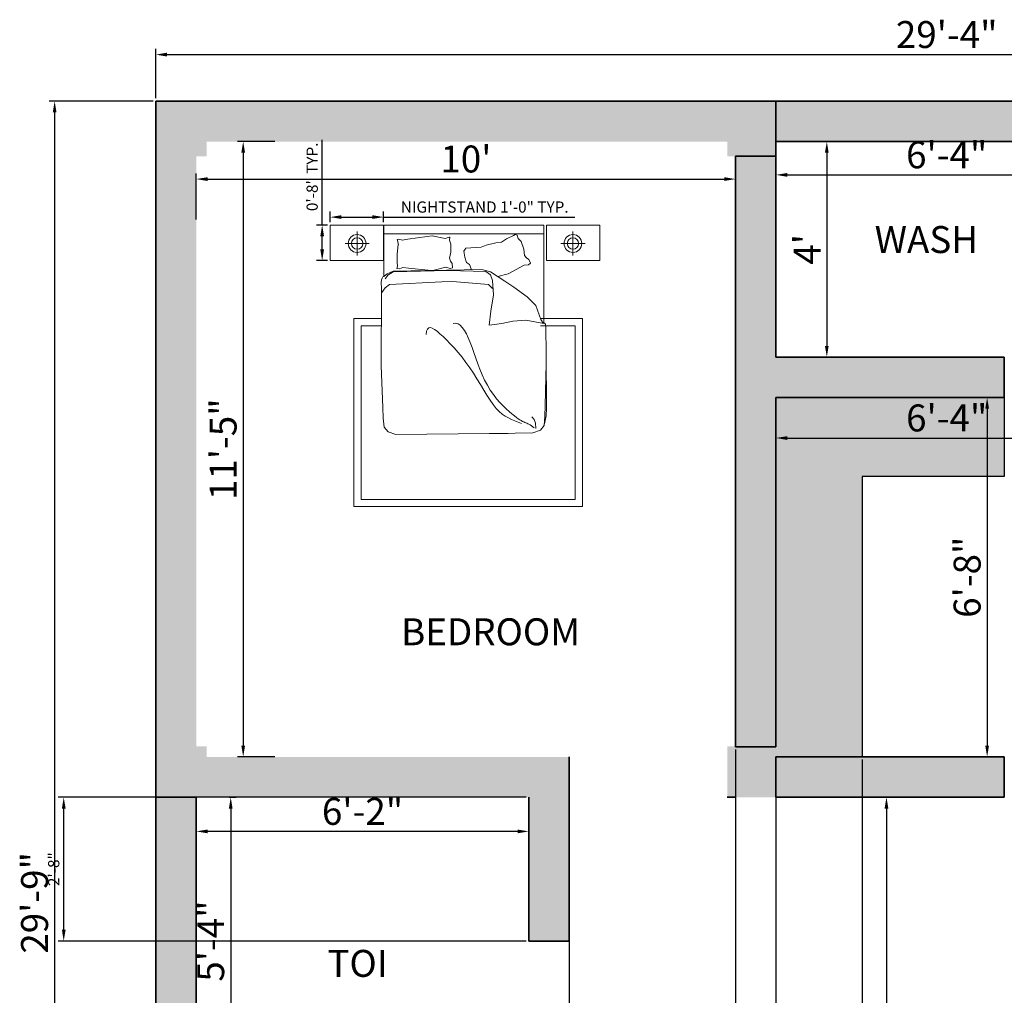
# Model space of a CAD drawing. Units: inches. Extents: x 3025 to 3429, y 1771 to 2198.
# Tile 2 of 3: x 3025 to 3244, y 1981 to 2198. Entities that reach past the tile are written whole.
import ezdxf

# ---------------------------------------------------------------- set-up
doc = ezdxf.new("R2010")
doc.units = ezdxf.units.IN
for name, color, linetype, lineweight in [('A-ANNO-DIMS', 2, 'Continuous', 18), ('A-AREA-IDEN', 7, 'Continuous', 25), ('A-COLS', 7, 'Continuous', 35), ('A-FLOR-FIXT', 9, 'Continuous', 25), ('A-FLOR-FIXT-PATT', 252, 'Continuous', 13), ('A-FURN', 8, 'Continuous', 18), ('A-WALL', 7, 'Continuous', 35), ('A-WALL-PATT', 3, 'Continuous', 13)]:
    doc.layers.add(name, color=color, linetype=linetype, lineweight=lineweight)
doc.layers.add('A-COLS-PATT', color=18, linetype='Continuous', lineweight=13, true_color=0x000000)
doc.styles.get("Standard").update_dxf_attribs({"font": 'arial.ttf'})
doc.dimstyles.new('ISO-25', dxfattribs={"dimtxt": 2.5, "dimasz": 2.5, "dimexe": 1.25, "dimexo": 0.625, "dimtad": 1, "dimdec": 0, "dimlunit": 3, "dimtxsty": 'Standard', "dimcen": 2.5, "dimadec": 0, "dimazin": 0, "dimtfac": 1, "dimtdec": 0, "dimtmove": 0, "dimatfit": 3, "dimfxl": 1, "dimarcsym": 0})

# ---------------------------------------------------------------- blocks, each defined once
blk = doc.blocks.new('*D1')
at = {"layer": 'A-ANNO-DIMS', "color": 0, "lineweight": -2, "transparency": 16777216}
for p, q in [((3054.93, 2180.84), (3054.93, 2191.81)), ((3406.93, 2180.84), (3406.93, 2191.81)), ((3057.43, 2190.56), (3404.43, 2190.56))]:
    blk.add_line(p, q, dxfattribs=at)
at = {"layer": 'A-ANNO-DIMS', "color": 0, "transparency": 16777216}
for points in [[(3057.43, 2190.98), (3057.43, 2190.14), (3054.93, 2190.56)], [(3404.43, 2190.98), (3404.43, 2190.14), (3406.93, 2190.56)]]:
    blk.add_solid(points, dxfattribs=at)
at = {"layer": 'Defpoints', "color": 0, "transparency": 16777216}
for p in [(3406.93, 2190.56), (3054.93, 2180.21), (3406.93, 2180.21)]:
    blk.add_point(p, dxfattribs=at)
at = {"layer": 'A-ANNO-DIMS', "color": 0, "transparency": 16777216, "insert": (3230.93, 2194.25), "char_height": 6, "attachment_point": 5}
blk.add_mtext('29\'-4"', dxfattribs=at)
blk = doc.blocks.new('*D2')
at = {"layer": 'A-ANNO-DIMS', "color": 0, "lineweight": -2, "transparency": 16777216}
for p, q in [((3071.28, 2025.21), (3072.84, 2025.21)), ((3071.59, 2022.71), (3071.59, 1963.71)), ((3071.28, 1961.21), (3072.84, 1961.21))]:
    blk.add_line(p, q, dxfattribs=at)
at = {"layer": 'A-ANNO-DIMS', "color": 0, "transparency": 16777216}
for points in [[(3071.17, 2022.71), (3072, 2022.71), (3071.59, 2025.21)], [(3071.17, 1963.71), (3072, 1963.71), (3071.59, 1961.21)]]:
    blk.add_solid(points, dxfattribs=at)
at = {"layer": 'Defpoints', "color": 0, "transparency": 16777216}
for p in [(3070.66, 2025.21), (3070.66, 1961.21), (3071.59, 1961.21)]:
    blk.add_point(p, dxfattribs=at)
at = {"layer": 'A-ANNO-DIMS', "color": 0, "transparency": 16777216, "insert": (3067.91, 1993.21), "char_height": 6, "attachment_point": 5, "rotation": 90}
blk.add_mtext('5\'-4"', dxfattribs=at)
blk = doc.blocks.new('*D3')
at = {"layer": 'A-ANNO-DIMS', "color": 0, "lineweight": -2, "transparency": 16777216}
for p, q in [((3063.93, 1994.3), (3063.93, 2018.87)), ((3137.93, 2006.87), (3137.93, 2018.87)), ((3135.43, 2017.62), (3066.43, 2017.62))]:
    blk.add_line(p, q, dxfattribs=at)
at = {"layer": 'A-ANNO-DIMS', "color": 0, "transparency": 16777216}
for points in [[(3066.43, 2018.03), (3066.43, 2017.2), (3063.93, 2017.62)], [(3135.43, 2018.03), (3135.43, 2017.2), (3137.93, 2017.62)]]:
    blk.add_solid(points, dxfattribs=at)
at = {"layer": 'Defpoints', "color": 0, "transparency": 16777216}
for p in [(3063.93, 2017.62), (3137.93, 2006.24), (3063.93, 1993.67)]:
    blk.add_point(p, dxfattribs=at)
at = {"layer": 'A-ANNO-DIMS', "color": 0, "transparency": 16777216, "insert": (3100.93, 2021.3), "char_height": 6, "attachment_point": 5}
blk.add_mtext('6\'-2"', dxfattribs=at)
blk = doc.blocks.new('*D6')
at = {"layer": 'A-ANNO-DIMS', "color": 0, "lineweight": -2, "transparency": 16777216}
for p, q in [((3081.41, 2171.21), (3073.12, 2171.21)), ((3074.37, 2168.71), (3074.37, 2036.71)), ((3081.41, 2034.21), (3073.12, 2034.21))]:
    blk.add_line(p, q, dxfattribs=at)
at = {"layer": 'A-ANNO-DIMS', "color": 0, "transparency": 16777216}
for points in [[(3073.95, 2168.71), (3074.78, 2168.71), (3074.37, 2171.21)], [(3073.95, 2036.71), (3074.78, 2036.71), (3074.37, 2034.21)]]:
    blk.add_solid(points, dxfattribs=at)
at = {"layer": 'Defpoints', "color": 0, "transparency": 16777216}
for p in [(3082.03, 2171.21), (3074.37, 2034.21), (3082.03, 2034.21)]:
    blk.add_point(p, dxfattribs=at)
at = {"layer": 'A-ANNO-DIMS', "color": 0, "transparency": 16777216, "insert": (3070.68, 2102.71), "char_height": 6, "attachment_point": 5, "rotation": 90}
blk.add_mtext('11\'-5"', dxfattribs=at)
blk = doc.blocks.new('*D7')
at = {"layer": 'A-ANNO-DIMS', "color": 0, "lineweight": -2, "transparency": 16777216}
for p, q in [((3063.93, 2153.83), (3063.93, 2164.1)), ((3066.43, 2162.85), (3181.43, 2162.85)), ((3183.93, 2145.67), (3183.93, 2164.1))]:
    blk.add_line(p, q, dxfattribs=at)
at = {"layer": 'A-ANNO-DIMS', "color": 0, "transparency": 16777216}
for points in [[(3066.43, 2163.26), (3066.43, 2162.43), (3063.93, 2162.85)], [(3181.43, 2163.26), (3181.43, 2162.43), (3183.93, 2162.85)]]:
    blk.add_solid(points, dxfattribs=at)
at = {"layer": 'Defpoints', "color": 0, "transparency": 16777216}
for p in [(3183.93, 2162.85), (3063.93, 2153.2), (3183.93, 2145.04)]:
    blk.add_point(p, dxfattribs=at)
at = {"layer": 'A-ANNO-DIMS', "color": 0, "transparency": 16777216, "insert": (3123.93, 2166.54), "char_height": 6, "attachment_point": 5}
blk.add_mtext("10'", dxfattribs=at)
blk = doc.blocks.new('*D8')
at = {"layer": 'A-ANNO-DIMS', "color": 0, "lineweight": -2, "transparency": 16777216}
for p, q in [((3205.85, 2171.21), (3203, 2171.21)), ((3204.25, 2168.71), (3204.25, 2125.71)), ((3205.85, 2123.21), (3203, 2123.21))]:
    blk.add_line(p, q, dxfattribs=at)
at = {"layer": 'A-ANNO-DIMS', "color": 0, "transparency": 16777216}
for points in [[(3203.83, 2168.71), (3204.66, 2168.71), (3204.25, 2171.21)], [(3203.83, 2125.71), (3204.66, 2125.71), (3204.25, 2123.21)]]:
    blk.add_solid(points, dxfattribs=at)
at = {"layer": 'Defpoints', "color": 0, "transparency": 16777216}
for p in [(3206.47, 2171.21), (3204.25, 2123.21), (3206.47, 2123.21)]:
    blk.add_point(p, dxfattribs=at)
at = {"layer": 'A-ANNO-DIMS', "color": 0, "transparency": 16777216, "insert": (3200.62, 2147.21), "char_height": 6, "attachment_point": 5, "rotation": 90}
blk.add_mtext("4'", dxfattribs=at)
blk = doc.blocks.new('*D9')
at = {"layer": 'A-ANNO-DIMS', "color": 0, "lineweight": -2, "transparency": 16777216}
for p, q in [((3192.93, 2164.54), (3192.93, 2162.53)), ((3195.43, 2163.78), (3266.43, 2163.78)), ((3268.93, 2164.54), (3268.93, 2162.53))]:
    blk.add_line(p, q, dxfattribs=at)
at = {"layer": 'A-ANNO-DIMS', "color": 0, "transparency": 16777216}
for points in [[(3195.43, 2164.2), (3195.43, 2163.37), (3192.93, 2163.78)], [(3266.43, 2164.2), (3266.43, 2163.37), (3268.93, 2163.78)]]:
    blk.add_solid(points, dxfattribs=at)
at = {"layer": 'Defpoints', "color": 0, "transparency": 16777216}
for p in [(3192.93, 2165.16), (3268.93, 2165.16), (3268.93, 2163.78)]:
    blk.add_point(p, dxfattribs=at)
at = {"layer": 'A-ANNO-DIMS', "color": 0, "transparency": 16777216, "insert": (3230.93, 2167.47), "char_height": 6, "attachment_point": 5}
blk.add_mtext('6\'-4"', dxfattribs=at)
blk = doc.blocks.new('*D12')
at = {"layer": 'A-ANNO-DIMS', "color": 0, "lineweight": -2, "transparency": 16777216}
for p, q in [((3054.31, 2180.21), (3031.16, 2180.21)), ((3032.41, 2177.71), (3032.41, 1825.71)), ((3054.31, 1823.21), (3031.16, 1823.21))]:
    blk.add_line(p, q, dxfattribs=at)
at = {"layer": 'A-ANNO-DIMS', "color": 0, "transparency": 16777216}
for points in [[(3031.99, 2177.71), (3032.82, 2177.71), (3032.41, 2180.21)], [(3031.99, 1825.71), (3032.82, 1825.71), (3032.41, 1823.21)]]:
    blk.add_solid(points, dxfattribs=at)
at = {"layer": 'Defpoints', "color": 0, "transparency": 16777216}
for p in [(3054.93, 2180.21), (3032.41, 1823.21), (3054.93, 1823.21)]:
    blk.add_point(p, dxfattribs=at)
at = {"layer": 'A-ANNO-DIMS', "color": 0, "transparency": 16777216, "insert": (3028.72, 2001.71), "char_height": 6, "attachment_point": 5, "rotation": 90}
blk.add_mtext('29\'-9"', dxfattribs=at)
blk = doc.blocks.new('*D14')
at = {"layer": 'A-ANNO-DIMS', "color": 0, "lineweight": -2, "transparency": 16777216}
for p, q in [((3227.77, 2114.21), (3241.17, 2114.21)), ((3239.92, 2111.71), (3239.92, 2036.71)), ((3227.77, 2034.21), (3241.17, 2034.21))]:
    blk.add_line(p, q, dxfattribs=at)
at = {"layer": 'A-ANNO-DIMS', "color": 0, "transparency": 16777216}
for points in [[(3239.51, 2111.71), (3240.34, 2111.71), (3239.92, 2114.21)], [(3239.51, 2036.71), (3240.34, 2036.71), (3239.92, 2034.21)]]:
    blk.add_solid(points, dxfattribs=at)
at = {"layer": 'Defpoints', "color": 0, "transparency": 16777216}
for p in [(3227.15, 2114.21), (3227.15, 2034.21), (3239.92, 2034.21)]:
    blk.add_point(p, dxfattribs=at)
at = {"layer": 'A-ANNO-DIMS', "color": 0, "transparency": 16777216, "insert": (3236.24, 2074.21), "char_height": 6, "attachment_point": 5, "rotation": 90}
blk.add_mtext('6\'-8"', dxfattribs=at)
blk = doc.blocks.new('*D15')
at = {"layer": 'A-ANNO-DIMS', "color": 0, "lineweight": -2, "transparency": 16777216}
for p, q in [((3192.93, 2097.44), (3192.93, 2106.45)), ((3268.93, 2098.84), (3268.93, 2106.45)), ((3195.43, 2105.2), (3266.43, 2105.2))]:
    blk.add_line(p, q, dxfattribs=at)
at = {"layer": 'A-ANNO-DIMS', "color": 0, "transparency": 16777216}
for points in [[(3195.43, 2105.61), (3195.43, 2104.78), (3192.93, 2105.2)], [(3266.43, 2105.61), (3266.43, 2104.78), (3268.93, 2105.2)]]:
    blk.add_solid(points, dxfattribs=at)
at = {"layer": 'Defpoints', "color": 0, "transparency": 16777216}
for p in [(3268.93, 2105.2), (3268.93, 2098.21), (3192.93, 2096.82)]:
    blk.add_point(p, dxfattribs=at)
at = {"layer": 'A-ANNO-DIMS', "color": 0, "transparency": 16777216, "insert": (3230.93, 2108.89), "char_height": 6, "attachment_point": 5}
blk.add_mtext('6\'-4"', dxfattribs=at)
blk = doc.blocks.new('*D17')
at = {"layer": 'A-ANNO-DIMS', "color": 0, "lineweight": -2, "transparency": 16777216}
for p, q in [((3225.75, 2025.21), (3216.27, 2025.21)), ((3217.52, 2022.71), (3217.52, 1910.71)), ((3225.75, 1908.21), (3216.27, 1908.21))]:
    blk.add_line(p, q, dxfattribs=at)
at = {"layer": 'A-ANNO-DIMS', "color": 0, "transparency": 16777216}
for points in [[(3217.1, 2022.71), (3217.94, 2022.71), (3217.52, 2025.21)], [(3217.1, 1910.71), (3217.94, 1910.71), (3217.52, 1908.21)]]:
    blk.add_solid(points, dxfattribs=at)
at = {"layer": 'Defpoints', "color": 0, "transparency": 16777216}
for p in [(3226.37, 2025.21), (3217.52, 1908.21), (3226.37, 1908.21)]:
    blk.add_point(p, dxfattribs=at)
at = {"layer": 'A-ANNO-DIMS', "color": 0, "transparency": 16777216, "insert": (3213.83, 1966.71), "char_height": 6, "attachment_point": 5, "rotation": 90}
blk.add_mtext('9\'-9"', dxfattribs=at)
blk = doc.blocks.new('NIGHTSTAND-12IN')
for p, q in [((6, 6.52), (6, 1.13)), ((3.31, 3.82), (8.69, 3.82))]:
    blk.add_line(p, q)
blk.add_lwpolyline([(0, 0), (11.88, 0), (11.88, 7.92), (0, 7.92)], close=True)
for radius in [1.98, 1.27]:
    blk.add_circle((6, 3.82), radius)
blk = doc.blocks.new('*D23')
at = {"layer": 'A-ANNO-DIMS', "color": 0, "lineweight": -2, "transparency": 16777216}
for p, q in [((3093.72, 2153.23), (3093.72, 2155.63)), ((3096.22, 2154.38), (3103.1, 2154.38)), ((3105.6, 2153.23), (3105.6, 2155.63)), ((3105.6, 2154.38), (3148.14, 2154.38))]:
    blk.add_line(p, q, dxfattribs=at)
at = {"layer": 'A-ANNO-DIMS', "color": 0, "transparency": 16777216}
for points in [[(3096.22, 2154.8), (3096.22, 2153.97), (3093.72, 2154.38)], [(3103.1, 2154.8), (3103.1, 2153.97), (3105.6, 2154.38)]]:
    blk.add_solid(points, dxfattribs=at)
at = {"layer": 'Defpoints', "color": 0, "transparency": 16777216}
for p in [(3105.6, 2154.38), (3093.72, 2152.6), (3105.6, 2152.6)]:
    blk.add_point(p, dxfattribs=at)
at = {"layer": 'A-ANNO-DIMS', "color": 0, "transparency": 16777216, "insert": (3128.12, 2156.3), "char_height": 2.5, "attachment_point": 5}
blk.add_mtext('NIGHTSTAND 1\'-0" TYP.', dxfattribs=at)
blk = doc.blocks.new('*D24')
at = {"layer": 'A-ANNO-DIMS', "color": 0, "lineweight": -2, "transparency": 16777216}
for p, q in [((3091.94, 2152.6), (3091.94, 2171.59)), ((3093.1, 2152.6), (3090.69, 2152.6)), ((3091.94, 2147.19), (3091.94, 2150.1)), ((3093.1, 2144.69), (3090.69, 2144.69))]:
    blk.add_line(p, q, dxfattribs=at)
at = {"layer": 'A-ANNO-DIMS', "color": 0, "transparency": 16777216}
for points in [[(3091.52, 2150.1), (3092.36, 2150.1), (3091.94, 2152.6)], [(3091.52, 2147.19), (3092.36, 2147.19), (3091.94, 2144.69)]]:
    blk.add_solid(points, dxfattribs=at)
at = {"layer": 'Defpoints', "color": 0, "transparency": 16777216}
for p in [(3091.94, 2152.6), (3093.72, 2152.6), (3093.72, 2144.69)]:
    blk.add_point(p, dxfattribs=at)
at = {"layer": 'A-ANNO-DIMS', "color": 0, "transparency": 16777216, "insert": (3090.04, 2163.35), "char_height": 2.5, "attachment_point": 5, "rotation": 90}
blk.add_mtext('0\'-8" TYP.', dxfattribs=at)
blk = doc.blocks.new('*D37')
at = {"layer": 'A-ANNO-DIMS', "color": 0, "lineweight": -2, "transparency": 16777216}
for p, q in [((3183.93, 2035.84), (3183.93, 1771.46)), ((3146.93, 2033.59), (3146.93, 1771.46)), ((3149.43, 1772.71), (3181.43, 1772.71))]:
    blk.add_line(p, q, dxfattribs=at)
at = {"layer": 'A-ANNO-DIMS', "color": 0, "transparency": 16777216}
for points in [[(3149.43, 1773.13), (3149.43, 1772.3), (3146.93, 1772.71)], [(3181.43, 1773.13), (3181.43, 1772.3), (3183.93, 1772.71)]]:
    blk.add_solid(points, dxfattribs=at)
at = {"layer": 'Defpoints', "color": 0, "transparency": 16777216}
for p in [(3183.93, 2036.47), (3146.93, 2034.21), (3183.93, 1772.71)]:
    blk.add_point(p, dxfattribs=at)
at = {"layer": 'A-ANNO-DIMS', "color": 0, "transparency": 16777216, "insert": (3165.43, 1774.62), "char_height": 2.5, "attachment_point": 5}
blk.add_mtext('3\'-1"', dxfattribs=at)
blk = doc.blocks.new('*D39')
at = {"layer": 'A-ANNO-DIMS', "color": 0, "lineweight": -2, "transparency": 16777216}
for p, q in [((3137.31, 2025.21), (3033.18, 2025.21)), ((3034.43, 1995.71), (3034.43, 2022.71)), ((3137.31, 1993.21), (3033.18, 1993.21))]:
    blk.add_line(p, q, dxfattribs=at)
at = {"layer": 'A-ANNO-DIMS', "color": 0, "transparency": 16777216}
for points in [[(3034.02, 2022.71), (3034.85, 2022.71), (3034.43, 2025.21)], [(3034.02, 1995.71), (3034.85, 1995.71), (3034.43, 1993.21)]]:
    blk.add_solid(points, dxfattribs=at)
at = {"layer": 'Defpoints', "color": 0, "transparency": 16777216}
for p in [(3034.43, 2025.21), (3137.93, 2025.21), (3137.93, 1993.21)]:
    blk.add_point(p, dxfattribs=at)
at = {"layer": 'A-ANNO-DIMS', "color": 0, "transparency": 16777216, "insert": (3032.53, 2009.21), "char_height": 2.5, "attachment_point": 5, "rotation": 90}
blk.add_mtext('2\'-8"', dxfattribs=at)
blk = doc.blocks.new('*D40')
at = {"layer": 'A-ANNO-DIMS', "color": 0, "lineweight": -2, "transparency": 16777216}
for p, q in [((3192.93, 2033.59), (3192.93, 1771.46)), ((3212.14, 2033.59), (3212.14, 1771.46)), ((3195.43, 1772.71), (3209.64, 1772.71))]:
    blk.add_line(p, q, dxfattribs=at)
at = {"layer": 'A-ANNO-DIMS', "color": 0, "transparency": 16777216}
for points in [[(3195.43, 1773.13), (3195.43, 1772.3), (3192.93, 1772.71)], [(3209.64, 1773.13), (3209.64, 1772.3), (3212.14, 1772.71)]]:
    blk.add_solid(points, dxfattribs=at)
at = {"layer": 'Defpoints', "color": 0, "transparency": 16777216}
for p in [(3192.93, 2034.21), (3212.14, 2034.21), (3212.14, 1772.71)]:
    blk.add_point(p, dxfattribs=at)
at = {"layer": 'A-ANNO-DIMS', "color": 0, "transparency": 16777216, "insert": (3202.54, 1774.59), "char_height": 2.5, "attachment_point": 5}
blk.add_mtext('1\'-7"', dxfattribs=at)

msp = doc.modelspace()

# ---------------------------------------------------------------- hatches: boundary and pattern name
at = {"layer": 'A-COLS-PATT'}
h = msp.add_hatch(color=256, dxfattribs=at)
h.dxf.hatch_style = 1
h.paths.add_polyline_path([(3066.27, 2180.21), (3054.93, 2180.21), (3054.93, 2167.95), (3063.93, 2167.95), (3063.93, 2171.21), (3066.27, 2171.21)])
h.paths.add_polyline_path([(3066.27, 2171.21), (3063.93, 2171.21), (3063.93, 2167.95), (3066.27, 2167.95)], flags=17)
h.paths.add_polyline_path([(3192.93, 2171.21), (3192.93, 2180.21), (3182.07, 2180.21), (3182.07, 2171.21), (3183.93, 2171.21), (3183.93, 2167.95), (3192.93, 2167.95)])
h.paths.add_polyline_path([(3183.93, 2171.21), (3182.07, 2171.21), (3182.07, 2167.95), (3183.93, 2167.95)], flags=17)
h = msp.add_hatch(color=256, dxfattribs=at)
h.dxf.hatch_style = 1
h.paths.add_polyline_path([(3066.27, 2034.21), (3063.93, 2034.21), (3063.93, 2036.54), (3054.93, 2036.54), (3054.93, 2025.21), (3063.93, 2025.21), (3066.27, 2025.21)])
h.paths.add_polyline_path([(3066.27, 2036.54), (3063.93, 2036.54), (3063.93, 2034.21), (3066.27, 2034.21)], flags=17)
h.paths.add_polyline_path([(3192.93, 2034.21), (3192.93, 2036.54), (3183.93, 2036.54), (3183.93, 2025.21), (3192.93, 2025.21)])
h = msp.add_hatch(color=256, dxfattribs=at)
h.dxf.hatch_style = 1
h.paths.add_polyline_path([(3183.93, 2036.54), (3182.07, 2036.54), (3182.07, 2025.21), (3183.93, 2025.21)])
at = {"layer": 'A-FLOR-FIXT-PATT'}
h = msp.add_hatch(dxfattribs=at)
h.set_pattern_fill('AR-CONC', color=256, scale=0.01)
h.paths.add_polyline_path([(3212.14, 2096.66), (3243.74, 2096.66), (3243.74, 2114.21), (3192.93, 2114.21), (3192.93, 2034.21), (3212.14, 2034.21)])
h.paths.add_polyline_path([(3221.13, 2102.65), (3240.82, 2102.65), (3240.82, 2115.01), (3221.13, 2115.01)], flags=9)
at = {"layer": 'A-WALL-PATT'}
h = msp.add_hatch(color=256, dxfattribs=at)
h.dxf.hatch_style = 1
h.paths.add_polyline_path([(3063.93, 1952.21), (3192.93, 1952.21), (3192.93, 1961.21), (3063.93, 1961.21), (3063.93, 2025.21), (3054.93, 2025.21), (3054.93, 1823.21), (3192.93, 1823.21), (3192.93, 1832.21), (3183.93, 1832.21), (3063.93, 1832.21)])
h.paths.add_polyline_path([(3146.93, 2034.21), (3063.93, 2034.21), (3063.93, 2036.54), (3054.93, 2036.54), (3054.93, 2025.21), (3063.93, 2025.21), (3137.93, 2025.21), (3137.93, 1993.21), (3146.93, 1993.21)])
h.paths.add_polyline_path([(3063.93, 2167.94), (3054.93, 2167.94), (3054.93, 2036.54), (3063.93, 2036.54)])
h.paths.add_polyline_path([(3182.07, 2180.21), (3066.24, 2180.21), (3066.24, 2171.21), (3182.07, 2171.21)])
h.paths.add_polyline_path([(3192.93, 2114.21), (3243.74, 2114.21), (3243.74, 2123.21), (3192.93, 2123.21), (3192.93, 2167.95), (3183.93, 2167.95), (3183.93, 2036.47), (3192.93, 2036.47)])
h = msp.add_hatch(color=256, dxfattribs=at)
h.dxf.hatch_style = 1
h.paths.add_polyline_path([(3268.93, 2180.21), (3192.93, 2180.21), (3192.93, 2171.21), (3268.93, 2171.21)])
h = msp.add_hatch(color=256, dxfattribs=at)
h.dxf.hatch_style = 1
h.paths.add_polyline_path([(3243.74, 2034.21), (3192.93, 2034.21), (3192.93, 2027.12), (3192.93, 2025.21), (3243.74, 2025.21)])

# ---------------------------------------------------------------- linework, layer by layer
at = {"layer": 'A-COLS'}
for p, q in [((3192.93, 2171.21), (3192.93, 2180.21)), ((3183.93, 2167.95), (3192.93, 2167.95)), ((3192.93, 2036.47), (3183.93, 2036.47)), ((3192.93, 2036.47), (3183.93, 2036.47)), ((3192.93, 2034.21), (3192.93, 2025.21)), ((3192.93, 2034.21), (3192.93, 2027.12)), ((3063.93, 2025.21), (3054.93, 2025.21)), ((3183.93, 2025.21), (3182.07, 2025.21))]:
    msp.add_line(p, q, dxfattribs=at)
at = {"layer": 'A-FLOR-FIXT'}
for p, q in [((3243.74, 2114.21), (3243.74, 2096.66)), ((3243.74, 2096.66), (3212.14, 2096.66)), ((3212.14, 2096.66), (3212.14, 2034.21))]:
    msp.add_line(p, q, dxfattribs=at)
at = {"layer": 'A-FURN'}
for p, q in [((3105.64, 2141.15), (3105.64, 2152.6)), ((3116.41, 2150.21), (3115.33, 2150.09)), ((3119.33, 2149.6), (3116.41, 2150.21)), ((3120.23, 2149.93), (3119.33, 2149.6)), ((3120.32, 2149.91), (3120.23, 2149.93)), ((3120.32, 2149.91), (3120.25, 2149.24)), ((3120.32, 2149.91), (3120.25, 2149.24)), ((3131.82, 2148.79), (3132.93, 2149.54)), ((3131.82, 2148.79), (3132.93, 2149.54)), ((3132.93, 2149.54), (3134.51, 2150.27)), ((3135.57, 2149.65), (3136.2, 2148.96)), ((3108.92, 2148.25), (3108.62, 2149.4)), ((3120.25, 2149.24), (3120.61, 2148.38)), ((3120.61, 2148.38), (3120.59, 2146.56)), ((3123.94, 2147.49), (3127.29, 2147.69)), ((3127.29, 2147.69), (3128.42, 2148.11)), ((3128.42, 2148.11), (3130.57, 2148.69)), ((3130.57, 2148.69), (3131.82, 2148.79)), ((3136.2, 2148.96), (3136.8, 2147.24)), ((3120.59, 2146.56), (3120.27, 2145.21)), ((3120.27, 2145.21), (3120.49, 2144.57)), ((3136.8, 2147.24), (3136.95, 2145.86)), ((3136.95, 2145.86), (3137.38, 2145.33)), ((3137.38, 2145.33), (3137.93, 2144.98)), ((3119.47, 2143.21), (3116.59, 2142.47)), ((3120.39, 2142.92), (3119.47, 2143.21)), ((3120.95, 2143.1), (3120.39, 2142.92)), ((3120.49, 2144.57), (3120.89, 2144.05)), ((3120.89, 2144.05), (3120.95, 2143.1)), ((3136.88, 2143.71), (3133.37, 2141.74)), ((3137.84, 2143.75), (3136.88, 2143.71)), ((3138.31, 2144.11), (3137.84, 2143.75)), ((3137.93, 2144.98), (3138.31, 2144.11)), ((3105.14, 2140.36), (3105.09, 2139.81)), ((3105.09, 2139.81), (3105.11, 2138.52)), ((3105.11, 2138.52), (3105.04, 2121.27)), ((3141.22, 2130.74), (3141.3, 2130.77)), ((3141.76, 2124.1), (3141.7, 2129.7)), ((3141.88, 2111.85), (3141.76, 2124.1)), ((3105.04, 2121.27), (3105.41, 2112.02)), ((3141.8, 2121.7), (3141.56, 2112.44)), ((3141.56, 2112.44), (3141.5, 2110.02)), ((3105.41, 2112.02), (3105.53, 2109.6)), ((3141.44, 2108.38), (3141.78, 2110.15)), ((3141.78, 2110.15), (3141.88, 2111.85)), ((3105.53, 2109.6), (3105.75, 2107.6)), ((3139.15, 2109.34), (3138.57, 2109.94)), ((3139.42, 2108.52), (3139.15, 2109.34)), ((3139.47, 2107.34), (3139.42, 2108.52)), ((3141.34, 2108.02), (3140.5, 2106.93)), ((3141.5, 2110.02), (3141.34, 2108.02)), ((3105.75, 2107.6), (3106.62, 2106.55)), ((3106.62, 2106.55), (3108.31, 2105.98)), ((3129.11, 2106.2), (3108.31, 2105.98)), ((3129.11, 2106.2), (3133.36, 2106.2)), ((3133.36, 2106.2), (3134.87, 2106.31)), ((3134.87, 2106.31), (3138.83, 2106.32)), ((3140.5, 2106.93), (3138.83, 2106.32))]:
    msp.add_line(p, q, dxfattribs=at)
for points in [[(3105.64, 2152.6), (3141.29, 2152.6), (3141.29, 2130.8)], [(3141.29, 2150.63), (3105.64, 2150.63)], [(3115.33, 2150.09), (3111.02, 2149.44), (3109.77, 2149.23), (3109.03, 2149.47), (3108.62, 2149.4)], [(3135.57, 2149.65), (3135.34, 2150.38), (3134.87, 2150.53), (3134.51, 2150.27)], [(3115.5, 2142.54), (3111.17, 2142.99), (3109.91, 2143.15), (3109.18, 2142.88), (3108.57, 2142.95), (3108.73, 2143.43), (3108.64, 2144.26), (3108.61, 2146.16), (3108.88, 2148.25)], [(3123.94, 2147.49), (3123.48, 2146.83), (3123.7, 2145.45), (3124.03, 2144.24), (3124.7, 2143.86), (3125.08, 2142.87), (3125.08, 2142.69)], [(3105.16, 2140.4), (3105.27, 2140.77), (3105.44, 2141.05), (3105.64, 2141.15), (3105.88, 2141.35), (3105.91, 2141.37)], [(3105.94, 2141.36), (3106.43, 2141.79), (3107.77, 2142.34), (3127.46, 2142.73), (3129.43, 2142.22), (3132.6, 2140.12), (3134.59, 2138.81), (3137.57, 2136.62), (3139.48, 2134.68), (3140.6, 2131.56), (3141.15, 2130.74)], [(3141.29, 2130.72), (3137.29, 2131.42), (3134.34, 2131.2), (3131.93, 2130.71), (3129.08, 2130.31), (3129.46, 2133.43), (3130.1, 2137.06), (3129.82, 2140.26), (3129.41, 2141.56), (3128.36, 2142.3), (3119.91, 2142.53), (3107.77, 2142.17), (3106.53, 2141.43), (3106, 2140.71), (3105.94, 2140.64)], [(3133.37, 2141.74), (3131.03, 2141.16)], [(3129.87, 2138.49), (3128.97, 2139.4), (3120.93, 2140.08), (3118.59, 2139.95), (3106.95, 2139.36), (3105.97, 2138.62), (3105.23, 2137.63)], [(3140.52, 2131.78), (3149.84, 2131.78), (3149.84, 2089.94), (3099.02, 2089.94), (3099.02, 2131.78), (3105.08, 2131.78)], [(3140.52, 2130.2), (3148.25, 2130.2), (3148.25, 2091.52), (3100.61, 2091.52), (3100.61, 2130.2), (3105.08, 2130.2)], [(3139.12, 2107.47), (3138.79, 2107.72), (3138.49, 2107.93), (3138.21, 2108.1), (3137.96, 2108.25), (3137.72, 2108.37), (3137.49, 2108.47), (3137.26, 2108.57), (3137.03, 2108.68), (3136.79, 2108.79), (3136.54, 2108.91), (3136.25, 2109.07), (3135.94, 2109.26), (3135.58, 2109.5), (3135.17, 2109.79), (3134.71, 2110.14), (3134.18, 2110.57), (3133.58, 2111.09), (3132.92, 2111.68), (3132.22, 2112.36), (3131.5, 2113.11), (3130.76, 2113.95), (3130.04, 2114.86), (3129.35, 2115.86), (3128.7, 2116.93), (3128.1, 2118.07), (3127.55, 2119.27), (3127.05, 2120.5), (3126.58, 2121.75), (3126.14, 2122.99), (3125.71, 2124.21), (3125.3, 2125.37), (3124.88, 2126.47), (3124.46, 2127.47), (3124.03, 2128.38), (3123.59, 2129.16), (3123.13, 2129.8), (3122.66, 2130.29), (3122.17, 2130.61), (3121.65, 2130.75), (3121.11, 2130.69)], [(3141.7, 2129.75), (3141.64, 2130.52), (3141.42, 2130.75), (3141.29, 2130.8)], [(3136.3, 2108.41), (3135.55, 2108.74), (3134.81, 2109.04), (3134.1, 2109.35), (3133.39, 2109.68), (3132.7, 2110.06), (3132.02, 2110.53), (3131.34, 2111.09), (3130.67, 2111.79), (3129.99, 2112.64), (3129.3, 2113.62), (3128.6, 2114.71), (3127.89, 2115.88), (3127.15, 2117.1), (3126.39, 2118.35), (3125.61, 2119.61), (3124.79, 2120.85), (3123.94, 2122.04), (3123.07, 2123.18), (3122.19, 2124.25), (3121.31, 2125.26), (3120.45, 2126.19), (3119.63, 2127.03), (3118.86, 2127.78), (3118.15, 2128.43), (3117.51, 2128.97), (3116.94, 2129.39), (3116.45, 2129.66), (3116.03, 2129.77), (3115.68, 2129.7), (3115.4, 2129.44), (3115.19, 2128.96), (3115.05, 2128.25)]]:
    msp.add_lwpolyline(points, dxfattribs=at)
at = {"layer": 'A-WALL'}
for p, q in [((3054.93, 2180.21), (3406.93, 2180.21)), ((3054.93, 2180.21), (3054.93, 1823.21)), ((3192.93, 2171.21), (3192.93, 2123.21)), ((3192.93, 2171.21), (3268.93, 2171.21)), ((3183.93, 2167.95), (3183.93, 2036.47)), ((3192.93, 2123.21), (3243.74, 2123.21)), ((3243.74, 2123.21), (3243.74, 2114.21)), ((3192.93, 2114.21), (3243.74, 2114.21)), ((3192.93, 2114.21), (3192.93, 2036.47)), ((3146.93, 2034.21), (3146.93, 1993.21)), ((3192.93, 2034.21), (3243.74, 2034.21)), ((3243.74, 2034.21), (3243.74, 2025.21)), ((3063.93, 2025.21), (3063.93, 1961.21)), ((3137.93, 2025.21), (3137.93, 1993.21)), ((3192.93, 2025.21), (3243.74, 2025.21)), ((3146.93, 1993.21), (3137.93, 1993.21))]:
    msp.add_line(p, q, dxfattribs=at)

# ---------------------------------------------------------------- block references
at = {"layer": 'A-FURN'}
msp.add_blockref('NIGHTSTAND-12IN', (3093.72, 2144.69), dxfattribs=at)
at = {"layer": 'A-FURN', "extrusion": (0, 0, -1), "zscale": -1}
msp.add_blockref('NIGHTSTAND-12IN', (-3153.75, 2144.69), dxfattribs=at)

# ---------------------------------------------------------------- texts
at = {"layer": 'A-AREA-IDEN', "char_height": 6, "attachment_point": 1}
for s, insert in [('WASH', (3214.9, 2152.38)), ('BEDROOM', (3109.51, 2065.06)), ('TOI', (3093.12, 1991.23))]:
    msp.add_mtext(s, dxfattribs=dict(at, insert=insert))

# ---------------------------------------------------------------- dimensions: what is measured, and where the dimension line sits
at = {"layer": 'A-ANNO-DIMS'}
for base, p1, p2, override, picture, middle in [((3406.93, 2190.56), (3054.93, 2180.21), (3406.93, 2180.21), {"dimtxt": 6, "dimclrd": 0, "dimclre": 0, "dimclrt": 0}, '*D1', (3230.93, 2194.25)), ((3268.93, 2163.78), (3192.93, 2165.16), (3268.93, 2165.16), {"dimtxt": 6, "dimclrd": 0, "dimclre": 0, "dimclrt": 0}, '*D9', (3230.93, 2167.47)), ((3183.93, 2162.85), (3063.93, 2153.2), (3183.93, 2145.04), {"dimtxt": 6, "dimclrd": 0, "dimclre": 0, "dimclrt": 0}, '*D7', (3123.93, 2166.54)), ((3268.93, 2105.2), (3192.93, 2096.82), (3268.93, 2098.21), {"dimtxt": 6, "dimclrd": 0, "dimclre": 0, "dimclrt": 0}, '*D15', (3230.93, 2108.89)), ((3183.93, 1772.71), (3146.93, 2034.21), (3183.93, 2036.47), {"dimdec": 1, "dimlfac": 1, "dimrnd": 0, "dimzin": 1, "dimdsep": 46, "dimlunit": 4, "dimfrac": 2}, '*D37', (3165.43, 1774.62)), ((3212.14, 1772.71), (3192.93, 2034.21), (3212.14, 2034.21), {"dimdec": 1, "dimlfac": 1, "dimrnd": 0, "dimzin": 1, "dimdsep": 46, "dimlunit": 4, "dimfrac": 2}, '*D40', (3202.54, 1774.59)), ((3063.93, 2017.62), (3137.93, 2006.24), (3063.93, 1993.67), {"dimtxt": 6, "dimclrd": 0, "dimclre": 0, "dimclrt": 0}, '*D3', (3100.93, 2021.3))]:
    dim = msp.add_linear_dim(base=base, p1=p1, p2=p2, dimstyle='ISO-25', override=override, dxfattribs=at)
    dim.commit()
    dim.dimension.update_dxf_attribs({"geometry": picture, "text_midpoint": middle})
for base, p1, p2, override, picture, middle in [((3032.41, 1823.21), (3054.93, 2180.21), (3054.93, 1823.21), {"dimtxt": 6, "dimclrd": 0, "dimclre": 0, "dimclrt": 0}, '*D12', (3028.72, 2001.71)), ((3074.37, 2034.21), (3082.03, 2171.21), (3082.03, 2034.21), {"dimtxt": 6, "dimclrd": 0, "dimclre": 0, "dimclrt": 0}, '*D6', (3070.68, 2102.71)), ((3204.25, 2123.21), (3206.47, 2171.21), (3206.47, 2123.21), {"dimtxt": 6, "dimclrd": 0, "dimclre": 0, "dimclrt": 0}, '*D8', (3200.62, 2147.21)), ((3239.92, 2034.21), (3227.15, 2114.21), (3227.15, 2034.21), {"dimtxt": 6, "dimclrd": 0, "dimclre": 0, "dimclrt": 0}, '*D14', (3236.24, 2074.21)), ((3034.43, 2025.21), (3137.93, 1993.21), (3137.93, 2025.21), {"dimdec": 1, "dimlfac": 1, "dimrnd": 0, "dimzin": 1, "dimdsep": 46, "dimlunit": 4, "dimfrac": 2}, '*D39', (3032.53, 2009.21)), ((3071.59, 1961.21), (3070.66, 2025.21), (3070.66, 1961.21), {"dimtxt": 6, "dimclrd": 0, "dimclre": 0, "dimclrt": 0}, '*D2', (3067.91, 1993.21)), ((3217.52, 1908.21), (3226.37, 2025.21), (3226.37, 1908.21), {"dimtxt": 6, "dimclrd": 0, "dimclre": 0, "dimclrt": 0}, '*D17', (3213.83, 1966.71))]:
    dim = msp.add_linear_dim(base=base, p1=p1, p2=p2, angle=90, dimstyle='ISO-25', override=override, dxfattribs=at)
    dim.commit()
    dim.dimension.update_dxf_attribs({"geometry": picture, "text_midpoint": middle})
dim = msp.add_linear_dim(base=(3091.94, 2152.6), p1=(3093.72, 2144.69), p2=(3093.72, 2152.6), angle=90, text='<> TYP.', dimstyle='ISO-25', override={"dimdec": 1, "dimlfac": 1, "dimrnd": 0, "dimzin": 1, "dimdsep": 46, "dimlunit": 4, "dimfrac": 2}, dxfattribs=at)
dim.commit()
dim.dimension.update_dxf_attribs({"geometry": '*D24', "text_midpoint": (3090.04, 2163.35)})
dim = msp.add_linear_dim(base=(3105.6, 2154.38), p1=(3093.72, 2152.6), p2=(3105.6, 2152.6), text='NIGHTSTAND <> TYP.', dimstyle='ISO-25', override={"dimdec": 1, "dimlfac": 1, "dimrnd": 0, "dimzin": 1, "dimdsep": 46, "dimlunit": 4, "dimfrac": 2}, dxfattribs=at)
dim.commit()
dim.dimension.update_dxf_attribs({"geometry": '*D23', "text_midpoint": (3128.12, 2156.3)})

doc.saveas('drawing.dxf')
